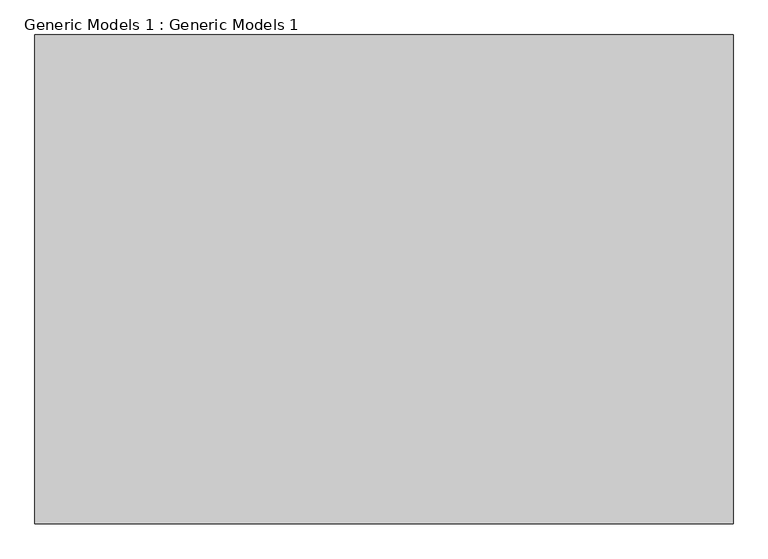
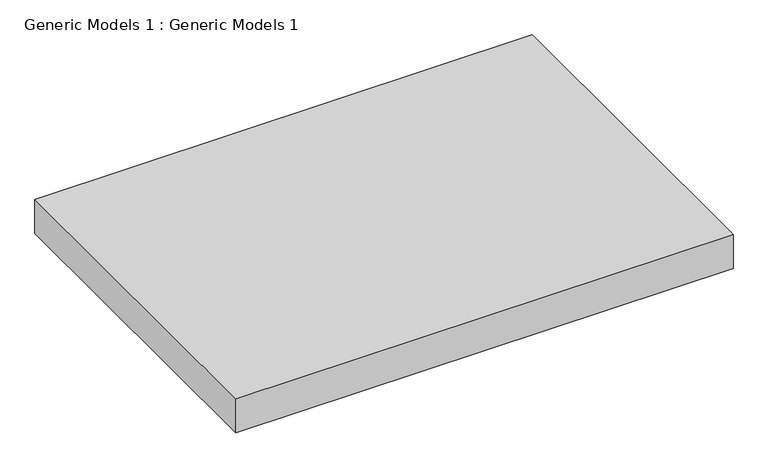
"""IFC4 building model written with IfcOpenShell, lengths in millimetres: proxy geometry, Generic Models 1 : Generic Models 1."""

from ifc_helpers import new_model, si_unit, origin, origin_with_axes, place, context, project, spatial, polyline, outline, extrude, source, transform, mapped, element, save


def generic_models_1_generic_models_1_86db66c4(model_context):
    return source(origin(), model_context, "Body", "SweptSolid", [
        extrude(outline(polyline([(-17432.2097681, -11313.0339922), (-17432.2097681, -14246.7339922), (-21623.2097681, -14246.7339922), (-21623.2097681, -11313.0339922), (-17432.2097681, -11313.0339922)])), origin_with_axes(), (0.0, 0.0, 1.0), 304.8),
    ])


if __name__ == "__main__":
    model = new_model("IFC4")
    model_context = context("Model", 3, world=origin())
    ifc_project = project(units=[si_unit("LENGTHUNIT", "METRE", prefix="MILLI")], contexts=[model_context])
    site = spatial("IfcSite", under=ifc_project)
    building = spatial("IfcBuilding", under=site)
    placement = place(None, origin())
    generic_models_1_generic_models_1_shape = generic_models_1_generic_models_1_86db66c4(model_context)
    element("IfcBuildingElementProxy", 1, Name="Generic Models 1 : Generic Models 1", ObjectType="Generic Models 1 : Generic Models 1", at=placement, inside=building, context=model_context, shape_type="MappedRepresentation", body=[
        mapped(generic_models_1_generic_models_1_shape, transform((0.0, 0.0, 0.0), x_axis=(1.0, 0.0, 0.0), y_axis=(0.0, 1.0, 0.0), z_axis=(0.0, 0.0, 1.0))),
    ])
    save(model, "model.ifc")
